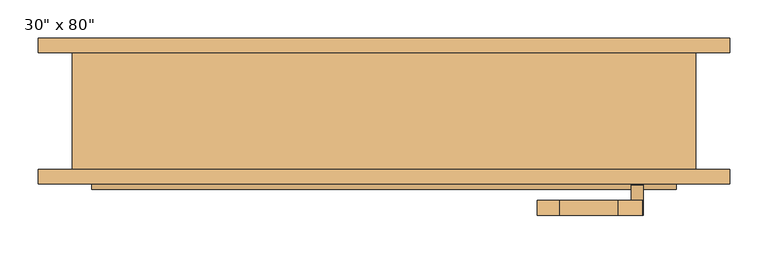
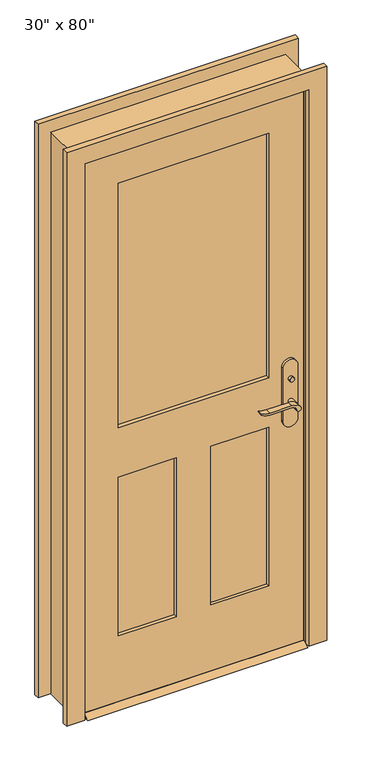
"""IFC4 building model written with IfcOpenShell, lengths in millimetres: door geometry."""

from ifc_helpers import new_model, si_unit, point, frame, frame_2d, origin, place, context, project, spatial, polyline, circle_curve, trimmed, segment, composite_curve, outline, extrude, faceted_brep, source, transform, mapped, element, save


def door_ce1fc124(model_context):
    return source(origin(), model_context, "Body", "SolidModel", [
        extrude(outline(polyline([(-38.1, 12.7), (-12.7, 0.0), (-98.425, 0.0), (-73.025, 12.7), (-38.1, 12.7)])), frame((-381.0, 0.0, 0.0), z_axis=(1.0, 0.0, 0.0), x_axis=(0.0, 1.0, 0.0)), (0.0, 0.0, 1.0), 762.0),
        extrude(outline(polyline([(335.2, -18.1), (335.2, -28.1), (325.2, -28.1), (325.2, -18.1), (335.2, -18.1)])), frame((0.0, 0.0, 981.9), z_axis=(0.0, 0.0, 1.0), x_axis=(1.0, 0.0, 0.0)), (0.0, 0.0, 1.0), 30.0),
        extrude(outline(composite_curve([segment(trimmed(circle_curve(frame_2d((996.9, 330.2)), 8.0), [point((996.9, 322.2))], [point((996.9, 338.2))], False, "CARTESIAN"), True, "CONTINUOUS"), segment(trimmed(circle_curve(frame_2d((996.9, 330.2)), 8.0), [point((996.9, 338.2))], [point((996.9, 322.2))], False, "CARTESIAN"), True, "CONTINUOUS")], self_intersect=False)), frame((0.0, -93.025, 0.0), z_axis=(0.0, 1.0, 0.0), x_axis=(0.0, 0.0, 1.0)), (0.0, 0.0, 1.0), 10.0),
        extrude(outline(composite_curve([segment(trimmed(circle_curve(frame_2d((897.1555521, 306.5324871)), 37.2832219), [point((919.0523287, 336.7081363))], [point((934.4, 304.8325667))], False, "CARTESIAN"), True, "CONTINUOUS"), segment(polyline([(934.4, 304.8325667), (934.4, 228.5564091)]), True, "CONTINUOUS"), segment(trimmed(circle_curve(frame_2d((1017.6850638, 228.6227909)), 83.2850902), [point((934.4, 228.5564091))], [point((939.4, 200.2))], True, "CARTESIAN"), True, "CONTINUOUS"), segment(polyline([(939.4, 200.2), (936.6135558, 200.2)]), True, "CONTINUOUS"), segment(trimmed(circle_curve(frame_2d((986.6709207, 232.1396612)), 59.3791355), [point((936.6135558, 200.2))], [point((927.4, 228.5564091))], False, "CARTESIAN"), True, "CONTINUOUS"), segment(polyline([(927.4, 228.5564091), (927.4, 304.8138099)]), True, "CONTINUOUS"), segment(trimmed(circle_curve(frame_2d((909.2738613, 304.8138099)), 18.1261387), [point((927.4, 304.8138099))], [point((914.4, 322.2))], True, "CARTESIAN"), True, "CONTINUOUS"), segment(trimmed(circle_curve(frame_2d((914.4, 330.2)), 8.0), [point((914.4, 322.2))], [point((919.0523287, 336.7081363))], False, "CARTESIAN"), True, "CONTINUOUS")], self_intersect=False)), frame((0.0, 1.9, 0.0), z_axis=(0.0, 1.0, 0.0), x_axis=(0.0, 0.0, 1.0)), (0.0, 0.0, 1.0), 20.0),
        extrude(outline(composite_curve([segment(trimmed(circle_curve(frame_2d((914.4, 330.2)), 8.0), [point((914.3999903, 322.2))], [point((919.0523287, 336.7081363))], False, "CARTESIAN"), True, "CONTINUOUS"), segment(trimmed(circle_curve(frame_2d((897.1555521, 306.5324871)), 37.2832219), [point((919.0523287, 336.7081363))], [point((934.4, 304.8325667))], False, "CARTESIAN"), True, "CONTINUOUS"), segment(polyline([(934.4, 304.8325667), (934.4, 228.5564091)]), True, "CONTINUOUS"), segment(trimmed(circle_curve(frame_2d((1017.6850638, 228.6227909)), 83.2850902), [point((934.4, 228.5564091))], [point((939.4, 200.2))], True, "CARTESIAN"), True, "CONTINUOUS"), segment(polyline([(939.4, 200.2), (936.6135558, 200.2)]), True, "CONTINUOUS"), segment(trimmed(circle_curve(frame_2d((986.6709207, 232.1396612)), 59.3791355), [point((936.6135558, 200.2))], [point((927.4, 228.5564091))], False, "CARTESIAN"), True, "CONTINUOUS"), segment(polyline([(927.4, 228.5564091), (927.4, 304.8138122)]), True, "CONTINUOUS"), segment(trimmed(circle_curve(frame_2d((909.2738682, 304.8138122)), 18.1261318), [point((927.4, 304.8138122))], [point((914.3999903, 322.2))], True, "CARTESIAN"), True, "CONTINUOUS")], self_intersect=False)), frame((0.0, -133.025, 0.0), z_axis=(0.0, 1.0, 0.0), x_axis=(0.0, 0.0, 1.0)), (0.0, 0.0, 1.0), 20.0),
        extrude(outline(composite_curve([segment(trimmed(circle_curve(frame_2d((914.4, 330.2)), 8.0), [point((914.4, 322.2))], [point((914.4, 338.2))], False, "CARTESIAN"), True, "CONTINUOUS"), segment(trimmed(circle_curve(frame_2d((914.4, 330.2)), 8.0), [point((914.4, 338.2))], [point((914.4, 322.2))], False, "CARTESIAN"), True, "CONTINUOUS")], self_intersect=False)), frame((0.0, -28.1, 0.0), z_axis=(0.0, 1.0, 0.0), x_axis=(0.0, 0.0, 1.0)), (0.0, 0.0, 1.0), 30.0),
        extrude(outline(composite_curve([segment(trimmed(circle_curve(frame_2d((914.4, 330.2)), 8.0), [point((914.4, 322.2))], [point((914.4, 338.2))], False, "CARTESIAN"), True, "CONTINUOUS"), segment(trimmed(circle_curve(frame_2d((914.4, 330.2)), 8.0), [point((914.4, 338.2))], [point((914.4, 322.2))], False, "CARTESIAN"), True, "CONTINUOUS")], self_intersect=False)), frame((0.0, -113.025, 0.0), z_axis=(0.0, 1.0, 0.0), x_axis=(0.0, 0.0, 1.0)), (0.0, 0.0, 1.0), 30.0),
        extrude(outline(composite_curve([segment(polyline([(844.4, 355.2), (1039.4, 355.2)]), True, "CONTINUOUS"), segment(trimmed(circle_curve(frame_2d((1039.4, 330.2)), 25.0), [point((1039.4, 355.2))], [point((1039.4, 305.2))], False, "CARTESIAN"), True, "CONTINUOUS"), segment(polyline([(1039.4, 305.2), (844.4, 305.2)]), True, "CONTINUOUS"), segment(trimmed(circle_curve(frame_2d((844.4, 330.2)), 25.0), [point((844.4, 305.2))], [point((844.4, 355.2))], False, "CARTESIAN"), True, "CONTINUOUS")], self_intersect=False)), frame((0.0, -38.1, 0.0), z_axis=(0.0, 1.0, 0.0), x_axis=(0.0, 0.0, 1.0)), (0.0, 0.0, 1.0), 10.0),
        extrude(outline(composite_curve([segment(polyline([(844.4, 355.2), (1039.4, 355.2)]), True, "CONTINUOUS"), segment(trimmed(circle_curve(frame_2d((1039.4, 330.2)), 25.0), [point((1039.4, 355.2))], [point((1039.4, 305.2))], False, "CARTESIAN"), True, "CONTINUOUS"), segment(polyline([(1039.4, 305.2), (844.4, 305.2)]), True, "CONTINUOUS"), segment(trimmed(circle_curve(frame_2d((844.4, 330.2)), 25.0), [point((844.4, 305.2))], [point((844.4, 355.2))], False, "CARTESIAN"), True, "CONTINUOUS")], self_intersect=False)), frame((0.0, -83.025, 0.0), z_axis=(0.0, 1.0, 0.0), x_axis=(0.0, 0.0, 1.0)), (0.0, 0.0, 1.0), 10.0),
        extrude(outline(polyline([(2032.0, -381.0), (12.7, -381.0), (12.7, 381.0), (2032.0, 381.0), (2032.0, -381.0)]), holes=[polyline([(1016.0, -260.35), (1911.35, -260.35), (1911.35, 260.35), (1016.0, 260.35), (1016.0, -260.35)]), polyline([(835.025, -60.325), (254.0, -60.325), (254.0, -260.35), (835.025, -260.35), (835.025, -60.325)]), polyline([(835.025, 260.35), (254.0, 260.35), (254.0, 60.325), (835.025, 60.325), (835.025, 260.35)])]), frame((0.0, -73.025, 0.0), z_axis=(0.0, 1.0, 0.0), x_axis=(0.0, 0.0, 1.0)), (0.0, 0.0, 1.0), 34.925),
        faceted_brep([(406.4, -73.025, 0.0), (381.0, -73.025, 0.0), (381.0, -38.1, 0.0), (368.3, -38.1, 0.0), (368.3, -3.175, 0.0), (381.0, -3.175, 0.0), (381.0, 79.375, 0.0), (406.4, 79.375, 0.0), (406.4, 79.375, 2057.4), (406.4, -73.025, 2057.4), (381.0, 79.375, 2032.0), (-381.0, 79.375, 2032.0), (-381.0, 79.375, 0.0), (-406.4, 79.375, 0.0), (-406.4, 79.375, 2057.4), (381.0, -3.175, 2032.0), (368.3, -3.175, 2019.3), (-368.3, -3.175, 2019.3), (-368.3, -3.175, 0.0), (-381.0, -3.175, 0.0), (-381.0, -3.175, 2032.0), (368.3, -38.1, 2019.3), (381.0, -38.1, 2032.0), (-381.0, -38.1, 2032.0), (-381.0, -38.1, 0.0), (-368.3, -38.1, 0.0), (-368.3, -38.1, 2019.3), (381.0, -73.025, 2032.0), (-406.4, -73.025, 2057.4), (-406.4, -73.025, 0.0), (-381.0, -73.025, 0.0), (-381.0, -73.025, 2032.0)], [[[0, 1, 2, 3, 4, 5, 6, 7]], [[7, 8, 9, 0]], [[6, 10, 11, 12, 13, 14, 8, 7]], [[5, 15, 10, 6]], [[4, 16, 17, 18, 19, 20, 15, 5]], [[3, 21, 16, 4]], [[2, 22, 23, 24, 25, 26, 21, 3]], [[1, 27, 22, 2]], [[0, 9, 28, 29, 30, 31, 27, 1]], [[8, 14, 28, 9]], [[15, 20, 11, 10]], [[21, 26, 17, 16]], [[27, 31, 23, 22]], [[29, 13, 12, 19, 18, 25, 24, 30]], [[14, 13, 29, 28]], [[20, 19, 12, 11]], [[26, 25, 18, 17]], [[31, 30, 24, 23]]]),
        extrude(outline(polyline([(-60.325, -49.7416667), (-60.325, -61.3833333), (-260.35, -61.3833333), (-260.35, -49.7416667), (-60.325, -49.7416667)])), frame((0.0, 0.0, 254.0), z_axis=(0.0, 0.0, 1.0), x_axis=(1.0, 0.0, 0.0)), (0.0, 0.0, 1.0), 581.025),
        extrude(outline(polyline([(260.35, -49.7416667), (260.35, -61.3833333), (60.325, -61.3833333), (60.325, -49.7416667), (260.35, -49.7416667)])), frame((0.0, 0.0, 254.0), z_axis=(0.0, 0.0, 1.0), x_axis=(1.0, 0.0, 0.0)), (0.0, 0.0, 1.0), 581.025),
        extrude(outline(polyline([(260.35, -52.07), (260.35, -59.055), (-260.35, -59.055), (-260.35, -52.07), (260.35, -52.07)])), frame((0.0, 0.0, 1016.0), z_axis=(0.0, 0.0, 1.0), x_axis=(1.0, 0.0, 0.0)), (0.0, 0.0, 1.0), 895.35),
        extrude(outline(polyline([(0.0, -387.35), (2038.35, -387.35), (2038.35, 387.35), (0.0, 387.35), (0.0, 450.85), (2101.85, 450.85), (2101.85, -450.85), (0.0, -450.85), (0.0, -387.35)])), frame((0.0, 79.375, 0.0), z_axis=(0.0, 1.0, 0.0), x_axis=(0.0, 0.0, 1.0)), (0.0, 0.0, 1.0), 19.05),
        extrude(outline(polyline([(0.0, -387.35), (2038.35, -387.35), (2038.35, 387.35), (0.0, 387.35), (0.0, 450.85), (2101.85, 450.85), (2101.85, -450.85), (0.0, -450.85), (0.0, -387.35)])), frame((0.0, -92.075, 0.0), z_axis=(0.0, 1.0, 0.0), x_axis=(0.0, 0.0, 1.0)), (0.0, 0.0, 1.0), 19.05),
    ])


if __name__ == "__main__":
    model = new_model("IFC4")
    model_context = context("Model", 3, world=origin())
    ifc_project = project(units=[si_unit("LENGTHUNIT", "METRE", prefix="MILLI")], contexts=[model_context])
    site = spatial("IfcSite", under=ifc_project)
    building = spatial("IfcBuilding", under=site)
    placement = place(None, origin())
    door_shape = door_ce1fc124(model_context)
    element("IfcDoor", 1, ObjectType="30\" x 80\"", at=placement, inside=building, context=model_context, shape_type="MappedRepresentation", body=[
        mapped(door_shape, transform((0.0, 0.0, 0.0), x_axis=(1.0, 0.0, 0.0), y_axis=(0.0, 1.0, 0.0), z_axis=(0.0, 0.0, 1.0))),
    ])
    save(model, "model.ifc")

# Revit data of these elements
# Type "30\" x 80\""
#   Type Mark = "9"
#   Assembly Code = "B2030100"
#   Analytic Construction = "French door, wood frame with single glass"
#   Top Rail = 0' - 4 3/4"
#   Threshold Offset [instance default] = 0' - 0 1/2"
#   Thickness = 0' - 1 3/8"
#   Thermal Resistance (R) = 1.0696 (h·ft²·°F)/BTU
#   Swing Angle [instance default] = 90.00°
#   Stiles = 0' - 4 3/4"
#   Rough Width = 2' - 8"
#   Rough Height = 6' - 9"
#   Lock Rail = 0' - 7 1/8"
#   Height = 6' - 8"
#   Width = 2' - 6"
#   Heat Transfer Coefficient (U) = 0.9350 BTU/(h·ft²·°F)
#   Door Offset [instance default] = 0' - 0"
#   Bottom Rail = 0' - 9 1/2"
#   Threshold [instance default] = yes
#   Function = 1
#   Exterior Trim [instance default] = yes
#   Trim Material = Cherry
#   Threshold Material = Cherry
#   Panel Material = Cherry
#   Glazing = Glass
#   Frame Material = Cherry
#   Door Handle Material = Aluminum
#   Visual Light Transmittance = 0
#   Solar Heat Gain Coefficient = 0
#   Wall Closure = (empty or 0)
#   Construction Type = (empty or 0)
# Element 1 (IfcDoor, "30\" x 80\"")
#   Materials on its faces: "Cherry", "Aluminum", "Glass"
# Materials
#   "Cherry": class "Wood", colour RGB 226 177 128, transparency 0, Description = "Prunus Serotina", Cost = 0
#   "Glass": class "Glass", colour RGB 0 128 192, transparency 0.75, Description = "Soda Lime Glass", Cost = 0
#   "Aluminum": class "Metal", colour RGB 247 247 247, transparency 0, Description = "Aluminum 6061", Cost = 0
